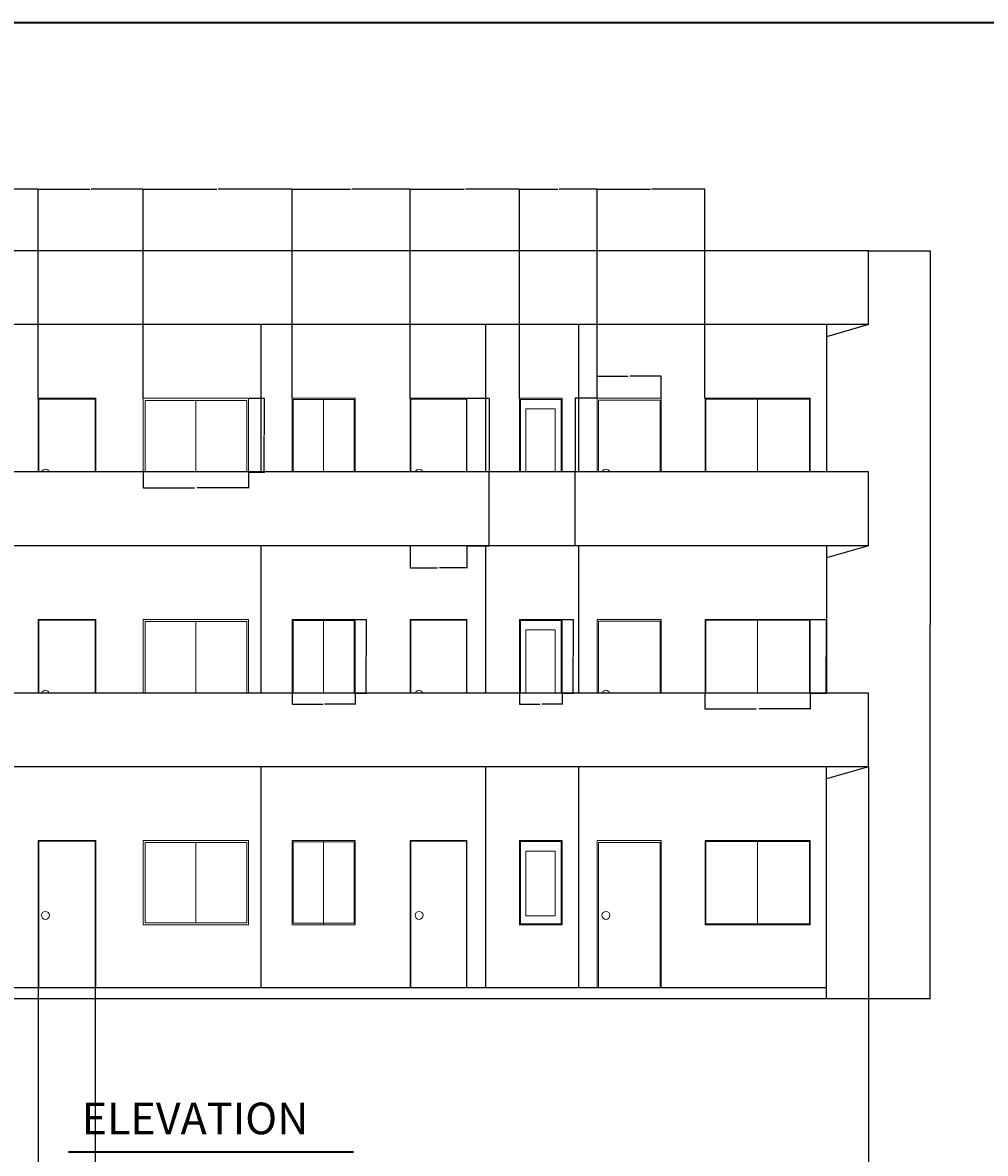
# Model space of a CAD drawing. Units: inches. Extents: x 1520 to 3401, y 1570 to 3432.
# Tile 9 of 15: x 1886 to 2435, y 2787 to 3432. Entities that reach past the tile are written whole.
import ezdxf

# ---------------------------------------------------------------- set-up
doc = ezdxf.new("R2010")
doc.units = ezdxf.units.IN
for name, color, linetype, lineweight in [('A-ANNO-DIMS', 2, 'Continuous', 18), ('A-ANNO-TITL', 7, 'Continuous', 35), ('A-ANNO-TTLB', 7, 'Continuous', 35), ('A-ELEV', 7, 'Continuous', 25), ('A-ELEV-DOOR', 3, 'Continuous', 18), ('A-ELEV-GLAZ', 4, 'Continuous', 18)]:
    doc.layers.add(name, color=color, linetype=linetype, lineweight=lineweight)
doc.styles.get("Standard").update_dxf_attribs({"font": 'arial.ttf'})
doc.dimstyles.get("Standard").update_dxf_attribs({"dimtxt": 0.18, "dimasz": 0.18, "dimexe": 0.18, "dimexo": 0.0625, "dimgap": 0.09, "dimtad": 0, "dimtih": 1, "dimtoh": 1, "dimdec": 4, "dimzin": 0, "dimdsep": 46, "dimtxsty": 'Standard', "dimcen": 0.09, "dimadec": 0, "dimazin": 0, "dimtfac": 1, "dimtdec": 4, "dimtofl": 0, "dimtmove": 0, "dimatfit": 3, "dimfxl": 1, "dimtolj": 1, "dimtzin": 0, "dimarcsym": 0})

# ---------------------------------------------------------------- blocks, each defined once
blk = doc.blocks.new('WIN-ELEV-04')
for p, q in [((0, 42), (0, 0)), ((60, 42), (0, 42)), ((0, 42), (0, 0)), ((60, 42), (0, 42)), ((30.07, 40.77), (30.07, 0)), ((60, 42), (60, 0)), ((60, 42), (60, 0))]:
    blk.add_line(p, q)
blk.add_lwpolyline([(1.08, 0), (1.08, 40.77), (59.06, 40.77), (59.06, 0)])
blk = doc.blocks.new('WIN-ELEV-05')
for p, q in [((0, 42), (0, 0)), ((36, 42), (0, 42)), ((0, 42), (0, 0)), ((36, 42), (0, 42)), ((17.94, 41.31), (17.94, 0)), ((36, 42), (36, 0)), ((36, 42), (36, 0))]:
    blk.add_line(p, q)
blk.add_lwpolyline([(0.56, 0), (0.56, 41.31), (35.32, 41.31), (35.32, 0)])
blk = doc.blocks.new('DOOR-ELEV-06')
for p, q in [((0, 84), (0, 42)), ((32.37, 84), (0, 84)), ((0, 84), (0, 42)), ((32.37, 84), (0, 84)), ((32.37, 84), (32.37, 42)), ((32.37, 84), (32.37, 42))]:
    blk.add_line(p, q)
for points in [[(0.35, 42), (0.35, 83.54), (32.06, 83.54), (32.06, 42)], [(32.06, 0), (32.06, 0), (0.35, 0)]]:
    blk.add_lwpolyline(points)
blk.add_arc((5.09, 41.3), 2.29, 17.89125, 162.10875)
blk = doc.blocks.new('WIN-ELEV-07')
for p, q in [((0, 42), (0, 0)), ((24.27, 42), (0, 42)), ((0, 42), (0, 0)), ((24.27, 42), (0, 42)), ((24.27, 42), (24.27, 0)), ((24.27, 42), (24.27, 0))]:
    blk.add_line(p, q)
for points in [[(0.51, 0), (0.51, 41.4), (23.72, 41.4), (23.72, 0)], [(3.54, 0), (3.54, 35.97), (20.19, 35.97), (20.19, 0)]]:
    blk.add_lwpolyline(points)
blk = doc.blocks.new('DOOR-ELEV-08')
for p, q in [((0, 84), (0, 42)), ((36.5, 84), (0, 84)), ((0, 84), (0, 42)), ((36.5, 84), (0, 84)), ((36.5, 84), (36.5, 42)), ((36.5, 84), (36.5, 42))]:
    blk.add_line(p, q)
for points in [[(0.75, 42), (0.75, 82.91), (35.79, 82.91), (35.79, 42)], [(35.79, 0), (0.75, 0)]]:
    blk.add_lwpolyline(points)
blk.add_arc((4.97, 41.3), 2.29, 17.89125, 162.10875)
blk = doc.blocks.new('WIN-ELEV-09')
for p, q in [((0, 42), (0, 0)), ((60, 42), (0, 42)), ((0, 42), (0, 0)), ((60, 42), (0, 42)), ((29.97, 41.48), (29.97, 0)), ((60, 42), (60, 0)), ((60, 42), (60, 0))]:
    blk.add_line(p, q)
blk.add_lwpolyline([(0.4, 0), (0.4, 41.48), (59.53, 41.48), (59.53, 0)])
blk = doc.blocks.new('*D161')
at = {"layer": 'A-ANNO-DIMS', "color": 0, "lineweight": -2, "transparency": 16777216}
for p, q in [((1954.64, 3175.57), (1954.64, 3166.45)), ((2014.64, 3175.57), (2014.64, 3166.45)), ((1954.82, 3166.63), (1983.81, 3166.63)), ((2014.46, 3166.63), (1985.47, 3166.63))]:
    blk.add_line(p, q, dxfattribs=at)
at = {"layer": 'A-ANNO-DIMS', "color": 0, "transparency": 16777216}
for points in [[(1954.82, 3166.66), (1954.82, 3166.6), (1954.64, 3166.63)], [(2014.46, 3166.66), (2014.46, 3166.6), (2014.64, 3166.63)]]:
    blk.add_solid(points, dxfattribs=at)
at = {"layer": 'Defpoints', "color": 0, "transparency": 16777216}
for p in [(1954.64, 3175.63), (2014.64, 3175.63), (2014.64, 3166.63)]:
    blk.add_point(p, dxfattribs=at)
at = {"layer": 'A-ANNO-DIMS', "color": 0, "transparency": 16777216, "insert": (1984.64, 3166.63), "char_height": 0.18, "attachment_point": 5}
blk.add_mtext('\\A1;EW4 60 TYP.', dxfattribs=at)
blk = doc.blocks.new('*D162')
at = {"layer": 'A-ANNO-DIMS', "color": 0, "lineweight": -2, "transparency": 16777216}
for p, q in [((2014.7, 3217.63), (2023.82, 3217.63)), ((2023.64, 3217.45), (2023.64, 3196.81)), ((2023.64, 3175.81), (2023.64, 3196.45)), ((2014.7, 3175.63), (2023.82, 3175.63))]:
    blk.add_line(p, q, dxfattribs=at)
at = {"layer": 'A-ANNO-DIMS', "color": 0, "transparency": 16777216}
for points in [[(2023.61, 3217.45), (2023.67, 3217.45), (2023.64, 3217.63)], [(2023.61, 3175.81), (2023.67, 3175.81), (2023.64, 3175.63)]]:
    blk.add_solid(points, dxfattribs=at)
at = {"layer": 'Defpoints', "color": 0, "transparency": 16777216}
for p in [(2014.64, 3217.63), (2023.64, 3217.63), (2014.64, 3175.63)]:
    blk.add_point(p, dxfattribs=at)
at = {"layer": 'A-ANNO-DIMS', "color": 0, "transparency": 16777216, "insert": (2023.64, 3196.63), "char_height": 0.18, "attachment_point": 5}
blk.add_mtext('\\A1;42 TYP.', dxfattribs=at)
blk = doc.blocks.new('*D163')
at = {"layer": 'A-ANNO-DIMS', "color": 0, "lineweight": -2, "transparency": 16777216}
for p, q in [((2075.56, 3091.63), (2081.97, 3091.63)), ((2081.79, 3091.45), (2081.79, 3070.81)), ((2081.79, 3049.81), (2081.79, 3070.45)), ((2075.56, 3049.63), (2081.97, 3049.63))]:
    blk.add_line(p, q, dxfattribs=at)
at = {"layer": 'A-ANNO-DIMS', "color": 0, "transparency": 16777216}
for points in [[(2081.76, 3091.45), (2081.82, 3091.45), (2081.79, 3091.63)], [(2081.76, 3049.81), (2081.82, 3049.81), (2081.79, 3049.63)]]:
    blk.add_solid(points, dxfattribs=at)
at = {"layer": 'Defpoints', "color": 0, "transparency": 16777216}
for p in [(2075.49, 3091.63), (2081.79, 3091.63), (2075.49, 3049.63)]:
    blk.add_point(p, dxfattribs=at)
at = {"layer": 'A-ANNO-DIMS', "color": 0, "transparency": 16777216, "insert": (2081.79, 3070.63), "char_height": 0.18, "attachment_point": 5}
blk.add_mtext('\\A1;EW5 42 TYP.', dxfattribs=at)
blk = doc.blocks.new('*D164')
at = {"layer": 'A-ANNO-DIMS', "color": 0, "lineweight": -2, "transparency": 16777216}
for p, q in [((2039.49, 3049.57), (2039.49, 3043.15)), ((2075.49, 3049.57), (2075.49, 3043.15)), ((2039.67, 3043.33), (2056.97, 3043.33)), ((2075.31, 3043.33), (2058.02, 3043.33))]:
    blk.add_line(p, q, dxfattribs=at)
at = {"layer": 'A-ANNO-DIMS', "color": 0, "transparency": 16777216}
for points in [[(2039.67, 3043.36), (2039.67, 3043.3), (2039.49, 3043.33)], [(2075.31, 3043.36), (2075.31, 3043.3), (2075.49, 3043.33)]]:
    blk.add_solid(points, dxfattribs=at)
at = {"layer": 'Defpoints', "color": 0, "transparency": 16777216}
for p in [(2039.49, 3049.63), (2075.49, 3049.63), (2075.49, 3043.33)]:
    blk.add_point(p, dxfattribs=at)
at = {"layer": 'A-ANNO-DIMS', "color": 0, "transparency": 16777216, "insert": (2057.49, 3043.33), "char_height": 0.18, "attachment_point": 5}
blk.add_mtext('\\A1;36 TYP.', dxfattribs=at)
blk = doc.blocks.new('*D165')
at = {"layer": 'A-ANNO-DIMS', "color": 0, "lineweight": -2, "transparency": 16777216}
for p, q in [((2139.24, 3217.63), (2151.95, 3217.63)), ((2151.77, 3217.45), (2151.77, 3175.81)), ((2151.77, 3133.81), (2151.77, 3175.45)), ((2139.24, 3133.63), (2151.95, 3133.63))]:
    blk.add_line(p, q, dxfattribs=at)
at = {"layer": 'A-ANNO-DIMS', "color": 0, "transparency": 16777216}
for points in [[(2151.74, 3217.45), (2151.8, 3217.45), (2151.77, 3217.63)], [(2151.74, 3133.81), (2151.8, 3133.81), (2151.77, 3133.63)]]:
    blk.add_solid(points, dxfattribs=at)
at = {"layer": 'Defpoints', "color": 0, "transparency": 16777216}
for p in [(2139.17, 3217.63), (2151.77, 3217.63), (2139.17, 3133.63)]:
    blk.add_point(p, dxfattribs=at)
at = {"layer": 'A-ANNO-DIMS', "color": 0, "transparency": 16777216, "insert": (2151.77, 3175.63), "char_height": 0.18, "attachment_point": 5}
blk.add_mtext('\\A1;ED6 84 TYP.', dxfattribs=at)
blk = doc.blocks.new('*D166')
at = {"layer": 'A-ANNO-DIMS', "color": 0, "lineweight": -2, "transparency": 16777216}
for p, q in [((2106.81, 3133.57), (2106.81, 3120.85)), ((2139.17, 3133.57), (2139.17, 3120.85)), ((2106.99, 3121.03), (2122.46, 3121.03)), ((2138.99, 3121.03), (2123.52, 3121.03))]:
    blk.add_line(p, q, dxfattribs=at)
at = {"layer": 'A-ANNO-DIMS', "color": 0, "transparency": 16777216}
for points in [[(2106.99, 3121.06), (2106.99, 3121), (2106.81, 3121.03)], [(2138.99, 3121.06), (2138.99, 3121), (2139.17, 3121.03)]]:
    blk.add_solid(points, dxfattribs=at)
at = {"layer": 'Defpoints', "color": 0, "transparency": 16777216}
for p in [(2106.81, 3133.63), (2139.17, 3133.63), (2139.17, 3121.03)]:
    blk.add_point(p, dxfattribs=at)
at = {"layer": 'A-ANNO-DIMS', "color": 0, "transparency": 16777216, "insert": (2122.99, 3121.03), "char_height": 0.18, "attachment_point": 5}
blk.add_mtext('\\A1;32 TYP.', dxfattribs=at)
blk = doc.blocks.new('*D167')
at = {"layer": 'A-ANNO-DIMS', "color": 0, "lineweight": -2, "transparency": 16777216}
for p, q in [((2193.56, 3091.63), (2199.98, 3091.63)), ((2199.8, 3091.45), (2199.8, 3070.81)), ((2199.8, 3049.81), (2199.8, 3070.45)), ((2193.56, 3049.63), (2199.98, 3049.63))]:
    blk.add_line(p, q, dxfattribs=at)
at = {"layer": 'A-ANNO-DIMS', "color": 0, "transparency": 16777216}
for points in [[(2199.77, 3091.45), (2199.83, 3091.45), (2199.8, 3091.63)], [(2199.77, 3049.81), (2199.83, 3049.81), (2199.8, 3049.63)]]:
    blk.add_solid(points, dxfattribs=at)
at = {"layer": 'Defpoints', "color": 0, "transparency": 16777216}
for p in [(2193.5, 3091.63), (2199.8, 3091.63), (2193.5, 3049.63)]:
    blk.add_point(p, dxfattribs=at)
at = {"layer": 'A-ANNO-DIMS', "color": 0, "transparency": 16777216, "insert": (2199.8, 3070.63), "char_height": 0.18, "attachment_point": 5}
blk.add_mtext('\\A1;EW7 42 TYP.', dxfattribs=at)
blk = doc.blocks.new('*D168')
at = {"layer": 'A-ANNO-DIMS', "color": 0, "lineweight": -2, "transparency": 16777216}
for p, q in [((2169.23, 3049.57), (2169.23, 3043.15)), ((2193.5, 3049.57), (2193.5, 3043.15)), ((2169.41, 3043.33), (2180.83, 3043.33)), ((2193.32, 3043.33), (2181.89, 3043.33))]:
    blk.add_line(p, q, dxfattribs=at)
at = {"layer": 'A-ANNO-DIMS', "color": 0, "transparency": 16777216}
for points in [[(2169.41, 3043.36), (2169.41, 3043.3), (2169.23, 3043.33)], [(2193.32, 3043.36), (2193.32, 3043.3), (2193.5, 3043.33)]]:
    blk.add_solid(points, dxfattribs=at)
at = {"layer": 'Defpoints', "color": 0, "transparency": 16777216}
for p in [(2169.23, 3049.63), (2193.5, 3049.63), (2193.5, 3043.33)]:
    blk.add_point(p, dxfattribs=at)
at = {"layer": 'A-ANNO-DIMS', "color": 0, "transparency": 16777216, "insert": (2181.36, 3043.33), "char_height": 0.18, "attachment_point": 5}
blk.add_mtext('\\A1;24 TYP.', dxfattribs=at)
blk = doc.blocks.new('*D169')
at = {"layer": 'A-ANNO-DIMS', "color": 0, "lineweight": -2, "transparency": 16777216}
for p, q in [((2213.39, 3217.63), (2200.67, 3217.63)), ((2200.85, 3217.45), (2200.85, 3175.81)), ((2200.85, 3133.81), (2200.85, 3175.45)), ((2213.39, 3133.63), (2200.67, 3133.63))]:
    blk.add_line(p, q, dxfattribs=at)
at = {"layer": 'A-ANNO-DIMS', "color": 0, "transparency": 16777216}
for points in [[(2200.82, 3217.45), (2200.88, 3217.45), (2200.85, 3217.63)], [(2200.82, 3133.81), (2200.88, 3133.81), (2200.85, 3133.63)]]:
    blk.add_solid(points, dxfattribs=at)
at = {"layer": 'Defpoints', "color": 0, "transparency": 16777216}
for p in [(2200.85, 3217.63), (2213.45, 3217.63), (2213.45, 3133.63)]:
    blk.add_point(p, dxfattribs=at)
at = {"layer": 'A-ANNO-DIMS', "color": 0, "transparency": 16777216, "insert": (2200.85, 3175.63), "char_height": 0.18, "attachment_point": 5}
blk.add_mtext('\\A1;ED8 84 TYP.', dxfattribs=at)
blk = doc.blocks.new('*D170')
at = {"layer": 'A-ANNO-DIMS', "color": 0, "lineweight": -2, "transparency": 16777216}
for p, q in [((2213.45, 3217.7), (2213.45, 3230.41)), ((2213.63, 3230.23), (2231.18, 3230.23)), ((2249.77, 3230.23), (2232.23, 3230.23)), ((2249.95, 3217.7), (2249.95, 3230.41))]:
    blk.add_line(p, q, dxfattribs=at)
at = {"layer": 'A-ANNO-DIMS', "color": 0, "transparency": 16777216}
for points in [[(2213.63, 3230.26), (2213.63, 3230.2), (2213.45, 3230.23)], [(2249.77, 3230.26), (2249.77, 3230.2), (2249.95, 3230.23)]]:
    blk.add_solid(points, dxfattribs=at)
at = {"layer": 'Defpoints', "color": 0, "transparency": 16777216}
for p in [(2249.95, 3230.23), (2213.45, 3217.63), (2249.95, 3217.63)]:
    blk.add_point(p, dxfattribs=at)
at = {"layer": 'A-ANNO-DIMS', "color": 0, "transparency": 16777216, "insert": (2231.7, 3230.23), "char_height": 0.18, "attachment_point": 5}
blk.add_mtext('\\A1;37 TYP.', dxfattribs=at)
blk = doc.blocks.new('*D171')
at = {"layer": 'A-ANNO-DIMS', "color": 0, "lineweight": -2, "transparency": 16777216}
for p, q in [((2274.88, 3049.57), (2274.88, 3040.45)), ((2334.88, 3049.57), (2334.88, 3040.45)), ((2275.06, 3040.63), (2304.05, 3040.63)), ((2334.7, 3040.63), (2305.72, 3040.63))]:
    blk.add_line(p, q, dxfattribs=at)
at = {"layer": 'A-ANNO-DIMS', "color": 0, "transparency": 16777216}
for points in [[(2275.06, 3040.66), (2275.06, 3040.6), (2274.88, 3040.63)], [(2334.7, 3040.66), (2334.7, 3040.6), (2334.88, 3040.63)]]:
    blk.add_solid(points, dxfattribs=at)
at = {"layer": 'Defpoints', "color": 0, "transparency": 16777216}
for p in [(2274.88, 3049.63), (2334.88, 3049.63), (2334.88, 3040.63)]:
    blk.add_point(p, dxfattribs=at)
at = {"layer": 'A-ANNO-DIMS', "color": 0, "transparency": 16777216, "insert": (2304.88, 3040.63), "char_height": 0.18, "attachment_point": 5}
blk.add_mtext('\\A1;EW9 60 TYP.', dxfattribs=at)
blk = doc.blocks.new('*D172')
at = {"layer": 'A-ANNO-DIMS', "color": 0, "lineweight": -2, "transparency": 16777216}
for p, q in [((2334.95, 3091.63), (2344.06, 3091.63)), ((2343.88, 3091.45), (2343.88, 3070.81)), ((2343.88, 3049.81), (2343.88, 3070.45)), ((2334.95, 3049.63), (2344.06, 3049.63))]:
    blk.add_line(p, q, dxfattribs=at)
at = {"layer": 'A-ANNO-DIMS', "color": 0, "transparency": 16777216}
for points in [[(2343.85, 3091.45), (2343.91, 3091.45), (2343.88, 3091.63)], [(2343.85, 3049.81), (2343.91, 3049.81), (2343.88, 3049.63)]]:
    blk.add_solid(points, dxfattribs=at)
at = {"layer": 'Defpoints', "color": 0, "transparency": 16777216}
for p in [(2334.88, 3091.63), (2343.88, 3091.63), (2334.88, 3049.63)]:
    blk.add_point(p, dxfattribs=at)
at = {"layer": 'A-ANNO-DIMS', "color": 0, "transparency": 16777216, "insert": (2343.88, 3070.63), "char_height": 0.18, "attachment_point": 5}
blk.add_mtext('\\A1;42 TYP.', dxfattribs=at)
blk = doc.blocks.new('*D209')
at = {"layer": 'A-ANNO-DIMS', "color": 0, "lineweight": -2, "transparency": 16777216}
for p, q in [((1675.61, 3007.57), (1675.61, 2752.86)), ((2368.11, 3007.57), (2368.11, 2752.86)), ((1675.79, 2753.04), (2021.47, 2753.04)), ((2367.93, 2753.04), (2022.26, 2753.04))]:
    blk.add_line(p, q, dxfattribs=at)
at = {"layer": 'A-ANNO-DIMS', "color": 0, "transparency": 16777216}
for points in [[(1675.79, 2753.07), (1675.79, 2753.01), (1675.61, 2753.04)], [(2367.93, 2753.07), (2367.93, 2753.01), (2368.11, 2753.04)]]:
    blk.add_solid(points, dxfattribs=at)
at = {"layer": 'Defpoints', "color": 0, "transparency": 16777216}
for p in [(1675.61, 3007.63), (2368.11, 3007.63), (2368.11, 2753.04)]:
    blk.add_point(p, dxfattribs=at)
at = {"layer": 'A-ANNO-DIMS', "color": 0, "transparency": 16777216, "insert": (2021.86, 2753.04), "char_height": 0.18, "attachment_point": 5}
blk.add_mtext('\\A1;692.5', dxfattribs=at)
blk = doc.blocks.new('*D210')
at = {"layer": 'A-ANNO-DIMS', "color": 0, "lineweight": -2, "transparency": 16777216}
for p, q in [((2368.18, 3301.63), (2403.39, 3301.63)), ((2403.21, 3301.45), (2403.21, 3088.81)), ((2403.21, 2875.81), (2403.21, 3088.45)), ((2344.18, 2875.63), (2403.39, 2875.63))]:
    blk.add_line(p, q, dxfattribs=at)
at = {"layer": 'A-ANNO-DIMS', "color": 0, "transparency": 16777216}
for points in [[(2403.18, 3301.45), (2403.24, 3301.45), (2403.21, 3301.63)], [(2403.18, 2875.81), (2403.24, 2875.81), (2403.21, 2875.63)]]:
    blk.add_solid(points, dxfattribs=at)
at = {"layer": 'Defpoints', "color": 0, "transparency": 16777216}
for p in [(2368.11, 3301.63), (2344.11, 2875.63), (2403.21, 2875.63)]:
    blk.add_point(p, dxfattribs=at)
at = {"layer": 'A-ANNO-DIMS', "color": 0, "transparency": 16777216, "insert": (2403.21, 3088.63), "char_height": 0.18, "attachment_point": 5}
blk.add_mtext('\\A1;426', dxfattribs=at)
blk = doc.blocks.new('*D214')
at = {"layer": 'A-ANNO-DIMS', "color": 0, "lineweight": -2, "transparency": 16777216}
for p, q in [((1894.73, 2881.57), (1894.73, 2752.86)), ((1927.22, 2881.57), (1927.22, 2752.86)), ((1894.91, 2753.04), (1910.58, 2753.04)), ((1927.04, 2753.04), (1911.37, 2753.04))]:
    blk.add_line(p, q, dxfattribs=at)
at = {"layer": 'A-ANNO-DIMS', "color": 0, "transparency": 16777216}
for points in [[(1894.91, 2753.07), (1894.91, 2753.01), (1894.73, 2753.04)], [(1927.04, 2753.07), (1927.04, 2753.01), (1927.22, 2753.04)]]:
    blk.add_solid(points, dxfattribs=at)
at = {"layer": 'Defpoints', "color": 0, "transparency": 16777216}
for p in [(1894.73, 2881.63), (1927.22, 2881.63), (1927.22, 2753.04)]:
    blk.add_point(p, dxfattribs=at)
at = {"layer": 'A-ANNO-DIMS', "color": 0, "transparency": 16777216, "insert": (1910.97, 2753.04), "char_height": 0.18, "attachment_point": 5}
blk.add_mtext('\\A1;32.49', dxfattribs=at)
blk = doc.blocks.new('*D217')
at = {"layer": 'A-ANNO-DIMS', "color": 0, "lineweight": -2, "transparency": 16777216}
for p, q in [((1845.96, 3217.7), (1845.96, 3336.91)), ((1846.14, 3336.73), (1869.94, 3336.73)), ((1894.55, 3336.73), (1870.74, 3336.73)), ((1894.73, 3217.7), (1894.73, 3336.91))]:
    blk.add_line(p, q, dxfattribs=at)
at = {"layer": 'A-ANNO-DIMS', "color": 0, "transparency": 16777216}
for points in [[(1846.14, 3336.76), (1846.14, 3336.7), (1845.96, 3336.73)], [(1894.55, 3336.76), (1894.55, 3336.7), (1894.73, 3336.73)]]:
    blk.add_solid(points, dxfattribs=at)
at = {"layer": 'Defpoints', "color": 0, "transparency": 16777216}
for p in [(1894.73, 3336.73), (1845.96, 3217.63), (1894.73, 3217.63)]:
    blk.add_point(p, dxfattribs=at)
at = {"layer": 'A-ANNO-DIMS', "color": 0, "transparency": 16777216, "insert": (1870.34, 3336.73), "char_height": 0.18, "attachment_point": 5}
blk.add_mtext('\\A1;48.77', dxfattribs=at)
blk = doc.blocks.new('*D218')
at = {"layer": 'A-ANNO-DIMS', "color": 0, "lineweight": -2, "transparency": 16777216}
for p, q in [((1894.73, 3217.7), (1894.73, 3336.91)), ((1894.91, 3336.73), (1924.31, 3336.73)), ((1954.46, 3336.73), (1925.06, 3336.73)), ((1954.64, 3217.7), (1954.64, 3336.91))]:
    blk.add_line(p, q, dxfattribs=at)
at = {"layer": 'A-ANNO-DIMS', "color": 0, "transparency": 16777216}
for points in [[(1894.91, 3336.76), (1894.91, 3336.7), (1894.73, 3336.73)], [(1954.46, 3336.76), (1954.46, 3336.7), (1954.64, 3336.73)]]:
    blk.add_solid(points, dxfattribs=at)
at = {"layer": 'Defpoints', "color": 0, "transparency": 16777216}
for p in [(1954.64, 3336.73), (1894.73, 3217.63), (1954.64, 3217.63)]:
    blk.add_point(p, dxfattribs=at)
at = {"layer": 'A-ANNO-DIMS', "color": 0, "transparency": 16777216, "insert": (1924.68, 3336.73), "char_height": 0.18, "attachment_point": 5}
blk.add_mtext('\\A1;59.91', dxfattribs=at)
blk = doc.blocks.new('*D219')
at = {"layer": 'A-ANNO-DIMS', "color": 0, "lineweight": -2, "transparency": 16777216}
for p, q in [((1954.64, 3217.7), (1954.64, 3336.91)), ((1954.82, 3336.73), (1996.67, 3336.73)), ((2039.31, 3336.73), (1997.46, 3336.73)), ((2039.49, 3217.7), (2039.49, 3336.91))]:
    blk.add_line(p, q, dxfattribs=at)
at = {"layer": 'A-ANNO-DIMS', "color": 0, "transparency": 16777216}
for points in [[(1954.82, 3336.76), (1954.82, 3336.7), (1954.64, 3336.73)], [(2039.31, 3336.76), (2039.31, 3336.7), (2039.49, 3336.73)]]:
    blk.add_solid(points, dxfattribs=at)
at = {"layer": 'Defpoints', "color": 0, "transparency": 16777216}
for p in [(2039.49, 3336.73), (1954.64, 3217.63), (2039.49, 3217.63)]:
    blk.add_point(p, dxfattribs=at)
at = {"layer": 'A-ANNO-DIMS', "color": 0, "transparency": 16777216, "insert": (1997.07, 3336.73), "char_height": 0.18, "attachment_point": 5}
blk.add_mtext('\\A1;84.85', dxfattribs=at)
blk = doc.blocks.new('*D220')
at = {"layer": 'A-ANNO-DIMS', "color": 0, "lineweight": -2, "transparency": 16777216}
for p, q in [((2039.49, 3217.7), (2039.49, 3336.91)), ((2039.67, 3336.73), (2072.77, 3336.73)), ((2106.63, 3336.73), (2073.53, 3336.73)), ((2106.81, 3217.7), (2106.81, 3336.91))]:
    blk.add_line(p, q, dxfattribs=at)
at = {"layer": 'A-ANNO-DIMS', "color": 0, "transparency": 16777216}
for points in [[(2039.67, 3336.76), (2039.67, 3336.7), (2039.49, 3336.73)], [(2106.63, 3336.76), (2106.63, 3336.7), (2106.81, 3336.73)]]:
    blk.add_solid(points, dxfattribs=at)
at = {"layer": 'Defpoints', "color": 0, "transparency": 16777216}
for p in [(2106.81, 3336.73), (2039.49, 3217.63), (2106.81, 3217.63)]:
    blk.add_point(p, dxfattribs=at)
at = {"layer": 'A-ANNO-DIMS', "color": 0, "transparency": 16777216, "insert": (2073.15, 3336.73), "char_height": 0.18, "attachment_point": 5}
blk.add_mtext('\\A1;67.31', dxfattribs=at)
blk = doc.blocks.new('*D221')
at = {"layer": 'A-ANNO-DIMS', "color": 0, "lineweight": -2, "transparency": 16777216}
for p, q in [((2106.81, 3217.7), (2106.81, 3336.91)), ((2106.99, 3336.73), (2137.62, 3336.73)), ((2169.05, 3336.73), (2138.41, 3336.73)), ((2169.23, 3217.7), (2169.23, 3336.91))]:
    blk.add_line(p, q, dxfattribs=at)
at = {"layer": 'A-ANNO-DIMS', "color": 0, "transparency": 16777216}
for points in [[(2106.99, 3336.76), (2106.99, 3336.7), (2106.81, 3336.73)], [(2169.05, 3336.76), (2169.05, 3336.7), (2169.23, 3336.73)]]:
    blk.add_solid(points, dxfattribs=at)
at = {"layer": 'Defpoints', "color": 0, "transparency": 16777216}
for p in [(2169.23, 3336.73), (2106.81, 3217.63), (2169.23, 3217.63)]:
    blk.add_point(p, dxfattribs=at)
at = {"layer": 'A-ANNO-DIMS', "color": 0, "transparency": 16777216, "insert": (2138.02, 3336.73), "char_height": 0.18, "attachment_point": 5}
blk.add_mtext('\\A1;62.42', dxfattribs=at)
blk = doc.blocks.new('*D222')
at = {"layer": 'A-ANNO-DIMS', "color": 0, "lineweight": -2, "transparency": 16777216}
for p, q in [((2169.23, 3217.7), (2169.23, 3336.91)), ((2169.41, 3336.73), (2190.94, 3336.73)), ((2213.27, 3336.73), (2191.74, 3336.73)), ((2213.45, 3217.7), (2213.45, 3336.91))]:
    blk.add_line(p, q, dxfattribs=at)
at = {"layer": 'A-ANNO-DIMS', "color": 0, "transparency": 16777216}
for points in [[(2169.41, 3336.76), (2169.41, 3336.7), (2169.23, 3336.73)], [(2213.27, 3336.76), (2213.27, 3336.7), (2213.45, 3336.73)]]:
    blk.add_solid(points, dxfattribs=at)
at = {"layer": 'Defpoints', "color": 0, "transparency": 16777216}
for p in [(2213.45, 3336.73), (2169.23, 3217.63), (2213.45, 3217.63)]:
    blk.add_point(p, dxfattribs=at)
at = {"layer": 'A-ANNO-DIMS', "color": 0, "transparency": 16777216, "insert": (2191.34, 3336.73), "char_height": 0.18, "attachment_point": 5}
blk.add_mtext('\\A1;44.23', dxfattribs=at)
blk = doc.blocks.new('*D223')
at = {"layer": 'A-ANNO-DIMS', "color": 0, "lineweight": -2, "transparency": 16777216}
for p, q in [((2213.45, 3217.7), (2213.45, 3336.91)), ((2213.63, 3336.73), (2243.78, 3336.73)), ((2274.7, 3336.73), (2244.56, 3336.73)), ((2274.88, 3217.7), (2274.88, 3336.91))]:
    blk.add_line(p, q, dxfattribs=at)
at = {"layer": 'A-ANNO-DIMS', "color": 0, "transparency": 16777216}
for points in [[(2213.63, 3336.76), (2213.63, 3336.7), (2213.45, 3336.73)], [(2274.7, 3336.76), (2274.7, 3336.7), (2274.88, 3336.73)]]:
    blk.add_solid(points, dxfattribs=at)
at = {"layer": 'Defpoints', "color": 0, "transparency": 16777216}
for p in [(2274.88, 3336.73), (2213.45, 3217.63), (2274.88, 3217.63)]:
    blk.add_point(p, dxfattribs=at)
at = {"layer": 'A-ANNO-DIMS', "color": 0, "transparency": 16777216, "insert": (2244.17, 3336.73), "char_height": 0.18, "attachment_point": 5}
blk.add_mtext('\\A1;61.43', dxfattribs=at)

msp = doc.modelspace()

# ---------------------------------------------------------------- linework, layer by layer
at = {"layer": 'A-ANNO-TITL'}
msp.add_line((1912.0951, 2788.1384), (2074.493, 2788.1384), dxfattribs=at)
at = {"layer": 'A-ANNO-TTLB'}
msp.add_lwpolyline([(1519.9253, 3431.7421), (3400.8761, 3431.7421), (3400.8761, 1570.3458), (1519.9253, 1570.3458)], close=True, dxfattribs=at)
at = {"layer": 'A-ELEV'}
for p, q in [((2368.1128, 3301.633), (1675.6128, 3301.633)), ((2368.1128, 3259.633), (2368.1128, 3301.633)), ((2368.1128, 3259.633), (1675.6128, 3259.633)), ((2021.8628, 3175.633), (2021.8628, 3259.633)), ((2150.0235, 3175.633), (2150.0235, 3259.633)), ((2203.0098, 3175.633), (2203.0098, 3259.633)), ((2344.1128, 3259.633), (2344.1128, 3175.633)), ((2368.1128, 3259.633), (2344.1128, 3252.6687)), ((2368.1128, 3175.633), (1675.6128, 3175.633)), ((2368.1128, 3133.633), (2368.1128, 3175.633)), ((2368.1128, 3133.633), (1675.6128, 3133.633)), ((2021.8628, 3049.633), (2021.8628, 3133.633)), ((2150.0235, 3049.633), (2150.0235, 3133.633)), ((2203.0098, 3049.633), (2203.0098, 3133.633)), ((2344.1128, 3133.633), (2344.1128, 3049.633)), ((2344.1128, 3133.633), (2344.1128, 3118.633)), ((2368.1128, 3133.633), (2344.1128, 3126.6687)), ((2368.1128, 3049.633), (1675.6128, 3049.633)), ((2368.1128, 3007.633), (2368.1128, 3049.633)), ((2368.1128, 3007.633), (1675.6128, 3007.633)), ((2021.8628, 2881.633), (2021.8628, 3007.633)), ((2150.0235, 2881.633), (2150.0235, 3007.633)), ((2203.0098, 2881.633), (2203.0098, 3007.633)), ((2344.1128, 2875.633), (2344.1128, 3007.633)), ((2368.1128, 3007.633), (2344.1128, 3000.6687)), ((2344.1128, 2881.633), (1699.6128, 2881.633)), ((1699.6128, 2875.633), (2344.1128, 2875.633))]:
    msp.add_line(p, q, dxfattribs=at)
at = {"layer": 'A-ELEV-DOOR'}
for p, q in [((1894.7277, 3217.633), (1894.7277, 3175.633)), ((1927.6174, 3217.633), (1894.7277, 3217.633)), ((1894.7277, 3217.633), (1894.7277, 3175.633)), ((1927.6174, 3217.633), (1894.7277, 3217.633)), ((1927.6174, 3217.633), (1927.6174, 3175.633)), ((1927.6174, 3217.633), (1927.6174, 3175.633)), ((1894.7277, 3091.633), (1894.7277, 3049.633)), ((1927.6174, 3091.633), (1894.7277, 3091.633)), ((1894.7277, 3091.633), (1894.7277, 3049.633)), ((1927.6174, 3091.633), (1894.7277, 3091.633)), ((1927.6174, 3091.633), (1927.6174, 3049.633)), ((1927.6174, 3091.633), (1927.6174, 3049.633)), ((1894.7277, 2965.633), (1894.7277, 2881.633)), ((1927.6174, 2965.633), (1894.7277, 2965.633)), ((1927.6174, 2965.633), (1927.6174, 2881.633)), ((2106.8084, 2965.633), (2106.8084, 2881.633)), ((2139.1737, 2965.633), (2106.8084, 2965.633)), ((2139.1737, 2965.633), (2139.1737, 2881.633)), ((2213.4538, 2965.633), (2213.4538, 2881.633)), ((2249.9544, 2965.633), (2213.4538, 2965.633)), ((2249.9544, 2965.633), (2249.9544, 2881.633))]:
    msp.add_line(p, q, dxfattribs=at)
for points in [[(1895.1743, 3175.633), (1895.1743, 3217.2074), (1927.2204, 3217.2074), (1927.2204, 3175.633)], [(1927.2204, 3133.633), (1895.1743, 3133.633)], [(1895.1743, 3049.633), (1895.1743, 3091.2074), (1927.2204, 3091.2074), (1927.2204, 3049.633)], [(1927.2204, 3007.633), (1927.2204, 3007.633), (1895.1743, 3007.633)]]:
    msp.add_lwpolyline(points, dxfattribs=at)
for points in [[(1895.1743, 2965.2074), (1927.2204, 2965.2074), (1927.2204, 2881.633), (1895.1743, 2881.633)], [(2107.1612, 2965.175), (2138.8684, 2965.175), (2138.8684, 2881.633), (2107.1612, 2881.633)], [(2214.2071, 2964.5466), (2249.2394, 2964.5466), (2249.2394, 2881.633), (2214.2071, 2881.633)]]:
    msp.add_lwpolyline(points, close=True, dxfattribs=at)
for centre in [(1898.8915, 2922.9304), (2111.9029, 2922.9304), (2218.4259, 2922.9304)]:
    msp.add_circle(centre, 2.2872, dxfattribs=at)
for centre in [(1898.8915, 3174.9304), (1898.8915, 3048.9304)]:
    msp.add_arc(centre, 2.2872, 17.8912507, 162.1087493, dxfattribs=at)
at = {"layer": 'A-ELEV-GLAZ'}
for p, q in [((1954.6418, 2965.633), (1954.6418, 2917.633)), ((2014.6418, 2965.633), (1954.6418, 2965.633)), ((2014.6418, 2965.633), (2014.6418, 2917.633)), ((2039.4942, 2965.633), (2039.4942, 2917.633)), ((2075.4942, 2965.633), (2039.4942, 2965.633)), ((2057.4339, 2964.9404), (2057.4339, 2917.633)), ((2075.4942, 2965.633), (2075.4942, 2917.633)), ((2169.2278, 2965.633), (2169.2278, 2917.633)), ((2193.4973, 2965.633), (2169.2278, 2965.633)), ((2193.4973, 2965.633), (2193.4973, 2917.633)), ((2274.885, 2965.633), (2274.885, 2917.633)), ((2334.885, 2965.633), (2274.885, 2965.633)), ((2304.8532, 2965.1123), (2304.8532, 2918.1231)), ((2334.885, 2965.633), (2334.885, 2917.633)), ((1984.7111, 2964.4075), (1984.7111, 2918.6643)), ((2014.6418, 2917.633), (1954.6418, 2917.633)), ((2075.4942, 2917.633), (2039.4942, 2917.633)), ((2193.4973, 2917.633), (2169.2278, 2917.633)), ((2334.885, 2917.633), (2274.885, 2917.633))]:
    msp.add_line(p, q, dxfattribs=at)
for points in [[(2040.0528, 2964.9404), (2074.815, 2964.9404), (2074.815, 2918.4097), (2040.0528, 2918.4097)], [(2169.737, 2965.0309), (2192.9519, 2965.0309), (2192.9519, 2918.075), (2169.737, 2918.075)], [(2275.2873, 2965.1123), (2334.4191, 2965.1123), (2334.4191, 2918.1231), (2275.2873, 2918.1231)], [(1955.7236, 2964.4075), (2013.6987, 2964.4075), (2013.6987, 2918.6643), (1955.7236, 2918.6643)], [(2172.7691, 2959.5992), (2189.4198, 2959.5992), (2189.4198, 2922.5918), (2172.7691, 2922.5918)]]:
    msp.add_lwpolyline(points, close=True, dxfattribs=at)

# ---------------------------------------------------------------- block references
at = {"layer": 'A-ELEV-DOOR'}
for name, p in [('DOOR-ELEV-06', (2106.808, 3133.633)), ('DOOR-ELEV-08', (2213.454, 3133.633)), ('DOOR-ELEV-06', (2106.808, 3007.633)), ('DOOR-ELEV-08', (2213.454, 3007.633))]:
    msp.add_blockref(name, p, dxfattribs=at)
at = {"layer": 'A-ELEV-GLAZ'}
for name, p in [('WIN-ELEV-04', (1954.642, 3175.633)), ('WIN-ELEV-05', (2039.494, 3175.633)), ('WIN-ELEV-07', (2169.228, 3175.633)), ('WIN-ELEV-09', (2274.885, 3175.633)), ('WIN-ELEV-04', (1954.642, 3049.633)), ('WIN-ELEV-05', (2039.494, 3049.633)), ('WIN-ELEV-07', (2169.228, 3049.633)), ('WIN-ELEV-09', (2274.885, 3049.633))]:
    msp.add_blockref(name, p, dxfattribs=at)

# ---------------------------------------------------------------- texts
at = {"layer": 'A-ANNO-TITL', "insert": (1919.5749, 2816.2081), "char_height": 18, "attachment_point": 1}
msp.add_mtext_dynamic_manual_height_columns('ELEVATION', width=373.373979, gutter_width=12.5, heights=[0], dxfattribs=at)

# ---------------------------------------------------------------- dimensions: what is measured, and where the dimension line sits
at = {"layer": 'A-ANNO-DIMS'}
for base, p1, p2, override, picture, middle in [((1894.7277, 3336.733), (1845.9552, 3217.633), (1894.7277, 3217.633), {"dimdec": 2, "dimlfac": 1, "dimrnd": 0, "dimzin": 0, "dimdsep": 46, "dimlunit": 2}, '*D217', (1870.3415, 3336.733)), ((1954.6418, 3336.733), (1894.7277, 3217.633), (1954.6418, 3217.633), {"dimdec": 2, "dimlfac": 1, "dimrnd": 0, "dimzin": 0, "dimdsep": 46, "dimlunit": 2}, '*D218', (1924.6847, 3336.733)), ((2039.4942, 3336.733), (1954.6418, 3217.633), (2039.4942, 3217.633), {"dimdec": 2, "dimlfac": 1, "dimrnd": 0, "dimzin": 0, "dimdsep": 46, "dimlunit": 2}, '*D219', (1997.068, 3336.733)), ((2106.8084, 3336.733), (2039.4942, 3217.633), (2106.8084, 3217.633), {"dimdec": 2, "dimlfac": 1, "dimrnd": 0, "dimzin": 0, "dimdsep": 46, "dimlunit": 2}, '*D220', (2073.1513, 3336.733)), ((2169.2278, 3336.733), (2106.8084, 3217.633), (2169.2278, 3217.633), {"dimdec": 2, "dimlfac": 1, "dimrnd": 0, "dimzin": 0, "dimdsep": 46, "dimlunit": 2}, '*D221', (2138.0181, 3336.733)), ((2213.4538, 3336.733), (2169.2278, 3217.633), (2213.4538, 3217.633), {"dimdec": 2, "dimlfac": 1, "dimrnd": 0, "dimzin": 0, "dimdsep": 46, "dimlunit": 2}, '*D222', (2191.3408, 3336.733)), ((2274.885, 3336.733), (2213.4538, 3217.633), (2274.885, 3217.633), {"dimdec": 2, "dimlfac": 1, "dimrnd": 0, "dimzin": 0, "dimdsep": 46, "dimlunit": 2}, '*D223', (2244.1694, 3336.733)), ((2368.1128, 2753.0384), (1675.6128, 3007.633), (2368.1128, 3007.633), {"dimdec": 1, "dimlfac": 1, "dimrnd": 0, "dimzin": 0, "dimdsep": 46, "dimlunit": 2}, '*D209', (2021.8628, 2753.0384)), ((1927.2204, 2753.0384), (1894.7277, 2881.633), (1927.2204, 2881.633), {"dimdec": 2, "dimlfac": 1, "dimrnd": 0, "dimzin": 0, "dimdsep": 46, "dimlunit": 2}, '*D214', (1910.9741, 2753.0384))]:
    dim = msp.add_linear_dim(base=base, p1=p1, p2=p2, dimstyle='Standard', override=override, dxfattribs=at)
    dim.commit()
    dim.dimension.update_dxf_attribs({"geometry": picture, "text_midpoint": middle})
dim = msp.add_linear_dim(base=(2403.2128, 2875.633), p1=(2368.1128, 3301.633), p2=(2344.1128, 2875.633), angle=90, dimstyle='Standard', override={"dimdec": 0, "dimlfac": 1, "dimrnd": 0, "dimzin": 0, "dimdsep": 46, "dimlunit": 2}, dxfattribs=at)
dim.commit()
dim.dimension.update_dxf_attribs({"geometry": '*D210', "text_midpoint": (2403.2128, 3088.633)})
for base, p1, p2, text, picture, middle in [((2249.9544, 3230.233), (2213.4538, 3217.633), (2249.9544, 3217.633), '<> TYP.', '*D170', (2231.7041, 3230.233)), ((2014.6418, 3166.633), (1954.6418, 3175.633), (2014.6418, 3175.633), 'EW4 <> TYP.', '*D161', (1984.6418, 3166.633)), ((2139.1737, 3121.033), (2106.8084, 3133.633), (2139.1737, 3133.633), '<> TYP.', '*D166', (2122.991, 3121.033)), ((2075.4942, 3043.333), (2039.4942, 3049.633), (2075.4942, 3049.633), '<> TYP.', '*D164', (2057.4942, 3043.333)), ((2193.4973, 3043.333), (2169.2278, 3049.633), (2193.4973, 3049.633), '<> TYP.', '*D168', (2181.3626, 3043.333)), ((2334.885, 3040.633), (2274.885, 3049.633), (2334.885, 3049.633), 'EW9 <> TYP.', '*D171', (2304.885, 3040.633))]:
    dim = msp.add_linear_dim(base=base, p1=p1, p2=p2, text=text, dimstyle='Standard', override={"dimdec": 0, "dimlfac": 1, "dimrnd": 0, "dimzin": 0, "dimdsep": 46, "dimlunit": 2}, dxfattribs=at)
    dim.commit()
    dim.dimension.update_dxf_attribs({"geometry": picture, "text_midpoint": middle})
for base, p1, p2, text, picture, middle in [((2023.6418, 3217.633), (2014.6418, 3175.633), (2014.6418, 3217.633), '<> TYP.', '*D162', (2023.6418, 3196.633)), ((2151.7737, 3217.633), (2139.1737, 3133.633), (2139.1737, 3217.633), 'ED6 <> TYP.', '*D165', (2151.7737, 3175.633)), ((2200.8538, 3217.633), (2213.4538, 3133.633), (2213.4538, 3217.633), 'ED8 <> TYP.', '*D169', (2200.8538, 3175.633)), ((2081.7942, 3091.633), (2075.4942, 3049.633), (2075.4942, 3091.633), 'EW5 <> TYP.', '*D163', (2081.7942, 3070.633)), ((2199.7973, 3091.633), (2193.4973, 3049.633), (2193.4973, 3091.633), 'EW7 <> TYP.', '*D167', (2199.7973, 3070.633)), ((2343.885, 3091.633), (2334.885, 3049.633), (2334.885, 3091.633), '<> TYP.', '*D172', (2343.885, 3070.633))]:
    dim = msp.add_linear_dim(base=base, p1=p1, p2=p2, angle=90, text=text, dimstyle='Standard', override={"dimdec": 0, "dimlfac": 1, "dimrnd": 0, "dimzin": 0, "dimdsep": 46, "dimlunit": 2}, dxfattribs=at)
    dim.commit()
    dim.dimension.update_dxf_attribs({"geometry": picture, "text_midpoint": middle})

doc.saveas('drawing.dxf')
